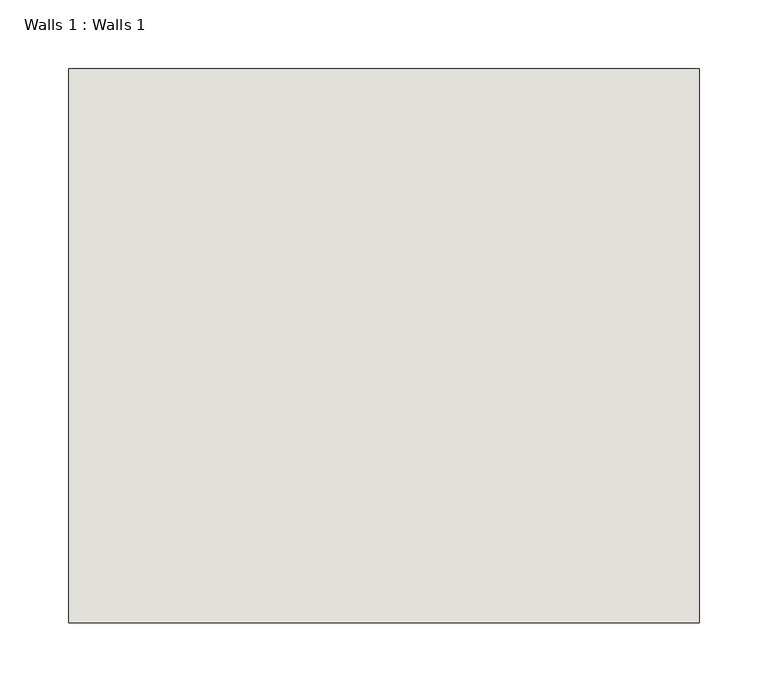
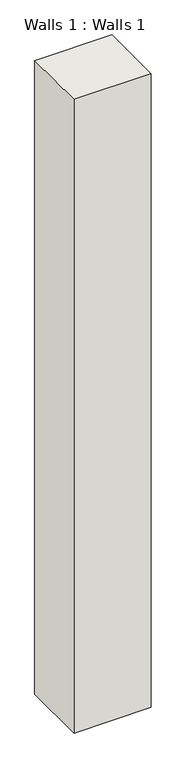
"""IFC4 building model written with IfcOpenShell, lengths in millimetres: wall geometry, Walls 1 : Walls 1."""

from ifc_helpers import new_model, si_unit, frame, origin, place, context, project, spatial, polyline, outline, extrude, source, transform, mapped, element, save


def walls_1_walls_1_ac2cf788(model_context):
    return source(origin(), model_context, "Body", "SweptSolid", [
        extrude(outline(polyline([(-8270.822521, -15855.5467593), (-8728.022521, -15855.5467593), (-8728.022521, -15453.751649), (-8270.822521, -15453.751649), (-8270.822521, -15855.5467593)])), frame((0.0, 0.0, 2895.6), z_axis=(0.0, 0.0, 1.0), x_axis=(1.0, 0.0, 0.0)), (0.0, 0.0, 1.0), 3962.4),
    ])


if __name__ == "__main__":
    model = new_model("IFC4")
    model_context = context("Model", 3, world=origin())
    ifc_project = project(units=[si_unit("LENGTHUNIT", "METRE", prefix="MILLI")], contexts=[model_context])
    site = spatial("IfcSite", under=ifc_project)
    building = spatial("IfcBuilding", under=site)
    placement = place(None, origin())
    walls_1_walls_1_shape = walls_1_walls_1_ac2cf788(model_context)
    element("IfcWall", 1, ObjectType="Walls 1 : Walls 1", at=placement, inside=building, context=model_context, shape_type="MappedRepresentation", body=[
        mapped(walls_1_walls_1_shape, transform((0.0, 0.0, 0.0), x_axis=(1.0, 0.0, 0.0), y_axis=(0.0, 1.0, 0.0), z_axis=(0.0, 0.0, 1.0))),
    ])
    save(model, "model.ifc")

# Revit data of these elements
# Element 1 (IfcWall, "Walls 1 : Walls 1")
#   Materials on its faces: "WALL-2 GREY", "Default Wall"
# Materials
#   "WALL-2 GREY": colour RGB 128 128 128, transparency 0, Cost = 0
#   "Default Wall": colour RGB 128 128 128, transparency 0
